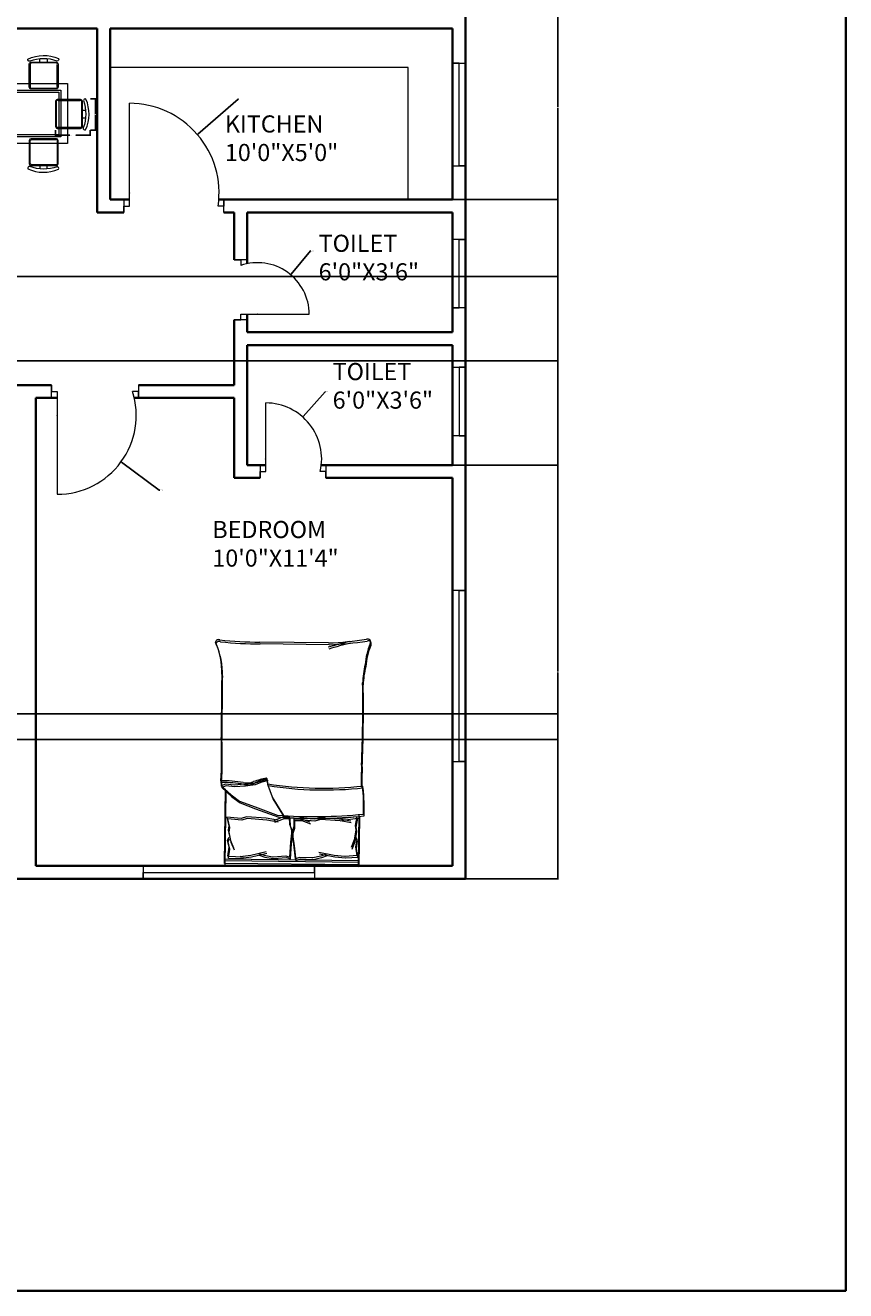
# Model space of a CAD drawing. Units: inches. Extents: x 1721 to 2510, y 1544 to 2360.
# Tile 5 of 10: x 2222 to 2510, y 1544 to 1988. Entities that reach past the tile are written whole.
import ezdxf

# ---------------------------------------------------------------- set-up
doc = ezdxf.new("R2010")
doc.units = ezdxf.units.IN
for name, color, linetype, lineweight in [('A-ANNO-DIMS', 2, 'Continuous', 18), ('A-ANNO-TTLB', 7, 'Continuous', 35), ('A-AREA-IDEN', 7, 'Continuous', 18), ('A-DOOR', 3, 'Continuous', 18), ('A-FLOR-FIXT', 9, 'Continuous', 18), ('A-FURN', 8, 'Continuous', 13), ('A-GLAZ', 4, 'Continuous', 18), ('A-WALL', 7, 'Continuous', 35)]:
    doc.layers.add(name, color=color, linetype=linetype, lineweight=lineweight)
doc.styles.get("Standard").update_dxf_attribs({"font": 'arial.ttf'})
doc.dimstyles.get("Standard").update_dxf_attribs({"dimtxt": 0.18, "dimasz": 0.18, "dimexe": 0.18, "dimexo": 0.0625, "dimgap": 0.09, "dimtad": 0, "dimtih": 1, "dimtoh": 1, "dimdec": 4, "dimzin": 0, "dimdsep": 46, "dimtxsty": 'Standard', "dimcen": 0.09, "dimadec": 0, "dimazin": 0, "dimtfac": 1, "dimtdec": 4, "dimtofl": 0, "dimtmove": 0, "dimatfit": 3, "dimfxl": 1, "dimtolj": 1, "dimtzin": 0, "dimarcsym": 0})

# ---------------------------------------------------------------- blocks, each defined once
blk = doc.blocks.new('BED-DOUBLE')
for p, q in [((39.64, 78.43), (15.52, 78.72)), ((39.64, 78.43), (15.52, 78.72)), ((39.86, 77.8), (15.74, 78.09)), ((39.86, 77.8), (15.74, 78.09)), ((1.93, 30.11), (1.99, 28.4, 3.79)), ((1.93, 30.11), (1.99, 28.4, 3.79)), ((3.5, 28.99), (1.99, 28.4)), ((3.5, 28.99), (1.99, 28.4)), ((1.99, 28.4), (5.58, 25.17)), ((1.99, 28.4), (5.58, 25.17)), ((2.15, 29.48), (2.21, 27.77, 3.79)), ((2.15, 29.48), (2.21, 27.77, 3.79)), ((3.72, 28.36), (2.21, 27.77)), ((3.72, 28.36), (2.21, 27.77)), ((2.21, 27.77), (5.8, 24.54)), ((2.21, 27.77), (5.8, 24.54)), ((3.23, 1.19), (3.55, 27.27)), ((3.23, 1.19), (3.55, 27.27)), ((3.45, 0.56), (3.76, 26.64)), ((3.45, 0.56), (3.76, 26.64)), ((6.54, 28.65), (3.5, 28.99)), ((6.54, 28.65), (3.5, 28.99)), ((6.75, 28.02), (3.72, 28.36)), ((6.75, 28.02), (3.72, 28.36)), ((10.33, 28.91), (6.54, 28.65)), ((10.33, 28.91), (6.54, 28.65)), ((10.55, 28.28), (6.75, 28.02)), ((10.55, 28.28), (6.75, 28.02)), ((13.68, 29.32), (10.33, 28.91)), ((13.68, 29.32), (10.33, 28.91)), ((13.89, 28.69), (10.55, 28.28)), ((13.89, 28.69), (10.55, 28.28)), ((15.66, 30.21), (13.68, 29.32)), ((15.66, 30.21), (13.68, 29.32)), ((15.88, 29.58), (13.89, 28.69)), ((15.88, 29.58), (13.89, 28.69)), ((18.1, 30.79), (15.66, 30.21)), ((18.1, 30.79), (15.66, 30.21)), ((18.31, 30.16), (15.88, 29.58)), ((18.31, 30.16), (15.88, 29.58)), ((18.38, 28.81), (18.1, 30.79)), ((18.38, 28.81), (18.1, 30.79)), ((18.59, 28.18), (18.31, 30.16)), ((18.59, 28.18), (18.31, 30.16)), ((20, 24.39), (18.38, 28.81)), ((20, 24.39), (18.38, 28.81)), ((20.21, 23.76), (18.59, 28.18)), ((20.21, 23.76), (18.59, 28.18)), ((5.58, 25.17), (8.44, 23.01)), ((5.58, 25.17), (8.44, 23.01)), ((5.8, 24.54), (8.66, 22.38)), ((5.8, 24.54), (8.66, 22.38)), ((8.44, 23.01), (13.88, 20.98)), ((8.44, 23.01), (13.88, 20.98)), ((8.66, 22.38), (14.1, 20.35)), ((8.66, 22.38), (14.1, 20.35)), ((24.03, 17.98), (20, 24.39)), ((24.03, 17.98), (20, 24.39)), ((24.24, 17.35), (20.21, 23.76)), ((24.24, 17.35), (20.21, 23.76)), ((13.88, 20.98), (22.02, 18)), ((13.88, 20.98), (22.02, 18)), ((14.1, 20.35), (22.24, 17.37)), ((14.1, 20.35), (22.24, 17.37)), ((50.28, 18.38), (50.07, 0.63)), ((50.28, 18.38), (50.07, 0.63)), ((50.5, 17.75), (50.29, 0)), ((50.5, 17.75), (50.29, 0)), ((9.01, 16.97), (3.98, 17.42)), ((3.98, 17.42), (4.71, 14.34)), ((9.01, 16.97), (3.98, 17.42)), ((3.98, 17.42), (4.71, 14.34)), ((9.23, 16.34), (4.2, 16.8)), ((4.2, 16.8), (4.92, 13.71)), ((9.23, 16.34), (4.2, 16.8)), ((4.2, 16.8), (4.92, 13.71)), ((4.71, 14.34), (4.5, 12.77)), ((4.71, 14.34), (4.5, 12.77)), ((4.92, 13.71), (4.72, 12.14)), ((4.92, 13.71), (4.72, 12.14)), ((10.94, 17.49), (9.01, 16.97)), ((10.94, 17.49), (9.01, 16.97)), ((11.15, 16.86), (9.23, 16.34)), ((11.15, 16.86), (9.23, 16.34)), ((17.8, 16.99), (10.94, 17.49)), ((17.8, 16.99), (10.94, 17.49)), ((18.02, 16.36), (11.15, 16.86)), ((18.02, 16.36), (11.15, 16.86)), ((21.75, 16.29), (17.8, 16.99)), ((21.75, 16.29), (17.8, 16.99)), ((21.96, 15.66), (18.02, 16.36)), ((21.96, 15.66), (18.02, 16.36)), ((23.54, 17.35), (20.51, 16.13)), ((23.54, 17.35), (20.51, 16.13)), ((23.75, 16.73), (20.73, 15.5)), ((23.75, 16.73), (20.73, 15.5)), ((25.94, 17.48), (23.54, 17.35)), ((25.94, 17.48), (23.54, 17.35)), ((26.16, 16.85), (23.75, 16.73)), ((26.16, 16.85), (23.75, 16.73)), ((26.07, 14.85), (25.94, 17.48)), ((26.07, 14.85), (25.94, 17.48)), ((26.73, 13.04), (26.07, 14.85)), ((26.73, 13.04), (26.07, 14.85)), ((26.29, 14.22), (26.16, 16.85)), ((26.29, 14.22), (26.16, 16.85)), ((26.95, 12.41), (26.29, 14.22)), ((26.95, 12.41), (26.29, 14.22)), ((27.02, 12.38), (27.61, 14.21)), ((27.02, 12.38), (27.61, 14.21)), ((27.23, 11.75), (27.82, 13.58)), ((27.23, 11.75), (27.82, 13.58)), ((27.61, 14.21), (27.64, 16.84)), ((27.61, 14.21), (27.64, 16.84)), ((27.64, 16.84), (30.05, 16.81)), ((27.64, 16.84), (30.05, 16.81)), ((27.82, 13.58), (27.85, 16.21)), ((27.82, 13.58), (27.85, 16.21)), ((27.85, 16.21), (30.26, 16.18)), ((27.85, 16.21), (30.26, 16.18)), ((34.67, 16.66), (29.65, 17.12)), ((34.67, 16.66), (29.65, 17.12)), ((34.89, 16.03), (29.86, 16.49)), ((34.89, 16.03), (29.86, 16.49)), ((30.05, 16.81), (33.11, 15.7)), ((30.05, 16.81), (33.11, 15.7)), ((30.26, 16.18), (33.33, 15.07)), ((30.26, 16.18), (33.33, 15.07)), ((36.6, 17.19), (34.67, 16.66)), ((36.6, 17.19), (34.67, 16.66)), ((36.81, 16.56), (34.89, 16.03)), ((36.81, 16.56), (34.89, 16.03)), ((43.46, 16.68), (36.6, 17.19)), ((43.46, 16.68), (36.6, 17.19)), ((43.68, 16.05), (36.81, 16.56)), ((43.68, 16.05), (36.81, 16.56)), ((43.46, 16.68), (44.58, 16.98)), ((43.46, 16.68), (44.58, 16.98)), ((47.41, 15.98), (43.46, 16.68)), ((47.41, 15.98), (43.46, 16.68)), ((43.68, 16.05), (44.79, 16.35)), ((43.68, 16.05), (44.79, 16.35)), ((47.62, 15.35), (43.68, 16.05)), ((47.62, 15.35), (43.68, 16.05)), ((44.58, 16.98), (49.58, 17.63)), ((44.58, 16.98), (49.58, 17.63)), ((44.79, 16.35), (49.8, 17)), ((44.79, 16.35), (49.8, 17)), ((49.58, 17.63), (48.98, 14.52)), ((49.58, 17.63), (48.98, 14.52)), ((48.98, 14.52), (49.24, 12.96)), ((48.98, 14.52), (49.24, 12.96)), ((49.8, 17), (49.19, 13.89)), ((49.8, 17), (49.19, 13.89)), ((49.19, 13.89), (49.46, 12.33)), ((49.19, 13.89), (49.46, 12.33)), ((4.25, 9.35), (4.77, 10.37)), ((4.25, 9.35), (4.77, 10.37)), ((4.8, 6.82), (4.25, 9.35)), ((4.8, 6.82), (4.25, 9.35)), ((4.47, 8.72), (4.98, 9.74)), ((4.47, 8.72), (4.98, 9.74)), ((4.5, 12.77), (5.25, 9.26)), ((4.5, 12.77), (5.25, 9.26)), ((4.72, 12.14), (5.46, 8.63)), ((4.72, 12.14), (5.46, 8.63)), ((5.25, 9.26), (6.37, 6.62)), ((5.25, 9.26), (6.37, 6.62)), ((26.39, 8.62), (26.8, 11.77)), ((26.39, 8.62), (26.8, 11.77)), ((26.61, 7.99), (27.01, 11.14)), ((26.61, 7.99), (27.01, 11.14)), ((26.8, 11.77), (26.73, 13.04)), ((26.8, 11.77), (26.73, 13.04)), ((27.01, 11.14), (26.95, 12.41)), ((27.01, 11.14), (26.95, 12.41)), ((27, 11.1), (27.02, 12.38)), ((27, 11.1), (27.02, 12.38)), ((27.53, 7.98), (27, 11.1)), ((27.53, 7.98), (27, 11.1)), ((27.22, 10.47), (27.23, 11.75)), ((27.22, 10.47), (27.23, 11.75)), ((27.75, 7.35), (27.22, 10.47)), ((27.75, 7.35), (27.22, 10.47)), ((48.63, 9.42), (47.61, 6.74)), ((48.63, 9.42), (47.61, 6.74)), ((49.24, 12.96), (48.63, 9.42)), ((49.24, 12.96), (48.63, 9.42)), ((49.46, 12.33), (48.85, 8.79)), ((49.46, 12.33), (48.85, 8.79)), ((49.63, 9.55), (49.07, 10.55)), ((49.63, 9.55), (49.07, 10.55)), ((49.17, 7.01), (49.63, 9.55)), ((49.17, 7.01), (49.63, 9.55)), ((49.84, 8.92), (49.29, 9.92)), ((49.84, 8.92), (49.29, 9.92)), ((49.39, 6.38), (49.84, 8.92)), ((49.39, 6.38), (49.84, 8.92)), ((4.39, 3.68), (4.8, 6.82)), ((4.39, 3.68), (4.8, 6.82)), ((5.02, 6.19), (4.47, 8.72)), ((5.02, 6.19), (4.47, 8.72)), ((4.61, 3.05), (5.02, 6.19)), ((4.61, 3.05), (5.02, 6.19)), ((5.46, 8.63), (6.59, 5.99)), ((5.46, 8.63), (6.59, 5.99)), ((12.44, 4.09), (17.76, 5.35)), ((12.44, 4.09), (17.76, 5.35)), ((12.65, 3.46), (17.98, 4.72)), ((12.65, 3.46), (17.98, 4.72)), ((15.1, 4.65), (17.12, 4.04)), ((15.1, 4.65), (17.12, 4.04)), ((26.09, 3.36), (26.39, 8.62)), ((26.09, 3.36), (26.39, 8.62)), ((26.3, 2.73), (26.61, 7.99)), ((26.3, 2.73), (26.61, 7.99)), ((28.04, 2.73), (27.53, 7.98)), ((28.04, 2.73), (27.53, 7.98)), ((28.25, 2.1), (27.75, 7.35)), ((28.25, 2.1), (27.75, 7.35)), ((41.65, 3.98), (36.28, 5.04)), ((41.65, 3.98), (36.28, 5.04)), ((38.96, 4.44), (36.97, 3.75)), ((38.96, 4.44), (36.97, 3.75)), ((48.85, 8.79), (47.82, 6.11)), ((48.85, 8.79), (47.82, 6.11)), ((49.7, 3.88), (49.17, 7.01)), ((49.7, 3.88), (49.17, 7.01)), ((49.92, 3.25), (49.39, 6.38)), ((49.92, 3.25), (49.39, 6.38)), ((50.07, 0.63), (3.23, 1.19)), ((50.07, 0.63), (3.23, 1.19)), ((50.09, 2.13), (3.25, 2.69)), ((50.09, 2.13), (3.25, 2.69)), ((50.29, 0), (3.45, 0.56)), ((50.29, 0), (3.45, 0.56)), ((50.31, 1.5), (3.47, 2.06)), ((50.31, 1.5), (3.47, 2.06)), ((4.39, 3.68), (9.69, 3.52)), ((4.39, 3.68), (9.69, 3.52)), ((4.61, 3.05), (9.9, 2.89)), ((4.61, 3.05), (9.9, 2.89)), ((8.71, 3.62), (12.44, 4.09)), ((8.71, 3.62), (12.44, 4.09)), ((9.69, 3.52), (8.71, 3.62)), ((9.69, 3.52), (8.71, 3.62)), ((8.92, 2.99), (12.65, 3.46)), ((8.92, 2.99), (12.65, 3.46)), ((9.9, 2.89), (8.92, 2.99)), ((9.9, 2.89), (8.92, 2.99)), ((15.32, 4.02), (17.34, 3.41)), ((15.32, 4.02), (17.34, 3.41)), ((17.12, 4.04), (19.98, 3.48)), ((17.12, 4.04), (19.98, 3.48)), ((17.34, 3.41), (20.2, 2.85)), ((17.34, 3.41), (20.2, 2.85)), ((19.98, 3.48), (20.3, 3.49)), ((19.98, 3.48), (20.3, 3.49)), ((20.2, 2.85), (20.52, 2.86)), ((20.2, 2.85), (20.52, 2.86)), ((20.3, 3.49), (24.64, 3.85)), ((20.3, 3.49), (24.64, 3.85)), ((20.52, 2.86), (24.86, 3.22)), ((20.52, 2.86), (24.86, 3.22)), ((24.64, 3.85), (26.09, 3.36)), ((24.64, 3.85), (26.09, 3.36)), ((24.86, 3.22), (26.3, 2.73)), ((24.86, 3.22), (26.3, 2.73)), ((29.46, 3.28), (28.04, 2.73)), ((29.46, 3.28), (28.04, 2.73)), ((29.68, 2.65), (28.25, 2.1)), ((29.68, 2.65), (28.25, 2.1)), ((33.81, 3.08), (29.46, 3.28)), ((33.81, 3.08), (29.46, 3.28)), ((34.03, 2.45), (29.68, 2.65)), ((34.03, 2.45), (29.68, 2.65)), ((34.13, 3.08), (33.81, 3.08)), ((34.13, 3.08), (33.81, 3.08)), ((34.35, 2.45), (34.03, 2.45)), ((34.35, 2.45), (34.03, 2.45)), ((36.97, 3.75), (34.13, 3.08)), ((36.97, 3.75), (34.13, 3.08)), ((37.19, 3.12), (34.35, 2.45)), ((37.19, 3.12), (34.35, 2.45)), ((41.87, 3.35), (36.49, 4.41)), ((41.87, 3.35), (36.49, 4.41)), ((39.18, 3.81), (37.19, 3.12)), ((39.18, 3.81), (37.19, 3.12)), ((45.39, 3.65), (41.65, 3.98)), ((45.39, 3.65), (41.65, 3.98)), ((45.61, 3.02), (41.87, 3.35)), ((45.61, 3.02), (41.87, 3.35)), ((45.5, 3.63), (45.39, 3.65)), ((45.5, 3.63), (45.39, 3.65)), ((49.7, 3.91), (45.5, 3.63)), ((49.7, 3.91), (45.5, 3.63)), ((45.71, 3), (45.61, 3.02)), ((45.71, 3), (45.61, 3.02)), ((49.91, 3.28), (45.71, 3)), ((49.91, 3.28), (45.71, 3))]:
    blk.add_line(p, q)
for centre, radius, start, end in [((1.08, 78.52), 1.08, 61.9736, 175.3348), ((1.08, 78.52), 1.08, 61.9736, 175.3348), ((-20.36, 68.78), 22.61, 356.7862, 25.7829), ((-20.36, 68.78), 22.61, 356.7862, 25.7829), ((1.29, 77.89), 1.08, 61.9736, 175.3348), ((1.29, 77.89), 1.08, 61.9736, 175.3348), ((-20.14, 68.15), 22.61, 356.7862, 25.7829), ((-20.14, 68.15), 22.61, 356.7862, 25.7829), ((15.63, 209.12), 130.4, 263.8146, 269.9499), ((15.63, 209.12), 130.4, 263.8146, 269.9499), ((15.85, 208.49), 130.4, 263.8146, 269.9499), ((15.85, 208.49), 130.4, 263.8146, 269.9499), ((70.08, -22.85), 104.34, 102.698, 107.0202), ((70.08, -22.85), 104.34, 102.698, 107.0202), ((34.83, 197.67), 119.34, 272.3106, 278.7239), ((34.83, 197.67), 119.34, 272.3106, 278.7239), ((70.29, -23.48), 104.34, 102.698, 107.0202), ((70.29, -23.48), 104.34, 102.698, 107.0202), ((35.05, 197.04), 119.34, 272.3106, 278.7239), ((35.05, 197.04), 119.34, 272.3106, 278.7239), ((75.53, 69.21), 23.09, 157.2899, 175.9668), ((75.53, 69.21), 23.09, 157.2899, 175.9668), ((75.75, 68.58), 23.09, 157.2899, 175.9668), ((75.75, 68.58), 23.09, 157.2899, 175.9668), ((53.35, 78.73), 1.07, 325.4884, 112.793), ((53.35, 78.73), 1.07, 325.4884, 112.793), ((53.56, 78.1), 1.07, 325.4884, 112.793), ((53.56, 78.1), 1.07, 325.4884, 112.793), ((4473.12, 14.21), 4471.22, 179.317, 179.60172), ((4473.12, 14.21), 4471.22, 179.317, 179.60172), ((4473.34, 13.58), 4471.22, 179.317, 179.60172), ((4473.34, 13.58), 4471.22, 179.317, 179.60172), ((80.6, 63.5), 29.05, 165.3797, 178.2261), ((80.6, 63.5), 29.05, 165.3797, 178.2261), ((80.81, 62.87), 29.05, 165.3797, 178.2261), ((80.81, 62.87), 29.05, 165.3797, 178.2261), ((-421.08, 55.88), 472.73, 357.5425, 1.0334), ((-421.08, 55.88), 472.73, 357.5425, 1.0334), ((-420.87, 55.25), 472.73, 357.5425, 1.0334), ((-420.87, 55.25), 472.73, 357.5425, 1.0334), ((-124.73, 38.32), 126.93, 356.294, 3.1513), ((-124.73, 38.32), 126.93, 356.294, 3.1513), ((-124.51, 37.69), 126.93, 356.294, 3.1513), ((-124.51, 37.69), 126.93, 356.294, 3.1513), ((217.81, 29.18), 166.73, 177.791, 180.323), ((217.81, 29.18), 166.73, 177.791, 180.323), ((218.03, 28.55), 166.73, 177.791, 180.323), ((218.03, 28.55), 166.73, 177.791, 180.323), ((3.1, -5.33), 35.46, 79.1911, 91.8805), ((3.1, -5.33), 35.46, 79.1911, 91.8805), ((3.31, -5.96), 35.46, 79.1911, 91.8805), ((3.31, -5.96), 35.46, 79.1911, 91.8805), ((11.02, 35.47), 6.1, 257.9756, 293.0532), ((11.02, 35.47), 6.1, 257.9756, 293.0532), ((11.23, 34.84), 6.1, 257.9756, 293.0532), ((11.23, 34.84), 6.1, 257.9756, 293.0532), ((22.96, 2.41), 29.06, 99.9765, 109.1954), ((22.96, 2.41), 29.06, 99.9765, 109.1954), ((23.18, 1.78), 29.06, 99.9765, 109.1954), ((23.18, 1.78), 29.06, 99.9765, 109.1954), ((17.93, 30.85), 0.181, 339.5612, 90.4525), ((17.93, 30.85), 0.181, 339.5612, 90.4525), ((18.15, 30.22), 0.181, 339.5612, 90.4525), ((18.15, 30.22), 0.181, 339.5612, 90.4525), ((37.91, 154), 126.46, 261.0993, 276.2154), ((37.91, 154), 126.46, 261.0993, 276.2154), ((38.12, 153.37), 126.46, 261.0993, 276.2154), ((38.12, 153.37), 126.46, 261.0993, 276.2154), ((-29.75, 21.28), 81.65, 358.0366, 4.9188), ((-29.75, 21.28), 81.65, 358.0366, 4.9188), ((-29.53, 20.65), 81.65, 358.0366, 4.9188), ((-29.53, 20.65), 81.65, 358.0366, 4.9188), ((34.68, 179.26), 161.69, 265.4014, 276.097), ((34.68, 179.26), 161.69, 265.4014, 276.097), ((34.89, 178.63), 161.69, 265.4014, 276.097), ((34.89, 178.63), 161.69, 265.4014, 276.097)]:
    blk.add_arc(centre, radius, start, end)
blk = doc.blocks.new('WIN-60IN-A')
for p, q in [((4.5, 60), (0, 60)), ((2.25, 0), (2.25, 60)), ((2.25, 60), (4.5, 60)), ((4.5, 0), (0, 0)), ((0, 0), (2.25, 0))]:
    blk.add_line(p, q)
blk = doc.blocks.new('WIN-24IN-A')
for p, q in [((4.5, 24), (0, 24)), ((0, 24), (2.25, 24)), ((2.25, 24), (2.25, 0)), ((4.5, 0), (0, 0)), ((2.25, 0), (4.5, 0))]:
    blk.add_line(p, q)
blk = doc.blocks.new('WIN-24IN-B')
for p, q in [((0, 24), (4.5, 24)), ((4.5, 24), (2.25, 24)), ((2.25, 24), (2.25, 0)), ((4.5, 0), (0, 0)), ((2.25, 0), (4.5, 0))]:
    blk.add_line(p, q)
blk = doc.blocks.new('WIN-60IN-B')
for p, q in [((2.25, 60), (0, 60)), ((0, 60), (4.5, 60)), ((2.25, 0), (2.25, 60)), ((4.5, 0), (0, 0)), ((0, 0), (2.25, 0))]:
    blk.add_line(p, q)
blk = doc.blocks.new('WIN-36IN-A')
for p, q in [((2.25, 36), (0, 36)), ((0, 36), (4.5, 36)), ((2.25, 0), (2.25, 36)), ((0, 0), (4.5, 0)), ((4.5, 0), (2.25, 0))]:
    blk.add_line(p, q)
blk = doc.blocks.new('TABLE-DINING-RECT')
for points in [[(0, 21.04), (35.07, 21.04), (35.07, 0), (0, 0)], [(2.34, 18.71), (32.73, 18.71), (32.73, 2.34), (2.34, 2.34)], [(3.04, 18), (32.03, 18), (32.03, 3.04), (3.04, 3.04)]]:
    blk.add_lwpolyline(points, close=True)
blk = doc.blocks.new('CHAIR-DINING-D')
for points in [[(0.75, 9.71, -0.578392), (0.03, 10.5, -0.214524), (10.81, 10.65, -0.552014), (10.31, 9.78, 0.175809), (0.75, 9.71)], [(10.03, 9.4, -0.414214), (10.65, 8.78), (10.65, 0.62, -0.414214), (10.03, 0), (1.16, 0, -0.414214), (0.54, 0.62), (0.54, 8.78, -0.414214), (1.16, 9.4), (10.03, 9.4)], [(4.27, 9.4), (4.27, 10.52, 0.064759)]]:
    blk.add_lwpolyline(points, format="xyb")
blk.add_lwpolyline([(10.02, 9.12), (1.44, 9.12, 0.414214), (0.82, 8.5), (0.82, 0.9, 0.414214), (1.44, 0.28), (10.02, 0.28, 0.512069), (10.37, 0.9), (10.37, 8.5, 0.512069)], format="xyb", close=True)
blk.add_lwpolyline([(6.76, 10.54), (6.76, 9.4)])
blk = doc.blocks.new('CHAIR-DINING-E')
for points in [[(9.4, 10.03, 0.414214), (8.77, 10.65), (0.62, 10.65, 0.414214), (0, 10.03), (0, 1.16, 0.414214), (0.62, 0.54), (8.77, 0.54, 0.414214), (9.4, 1.16), (9.4, 10.03)], [(9.78, 10.31, -0.175809), (9.71, 0.75, 0.578392), (10.5, 0.03, 0.214524), (10.65, 10.81, 0.552014), (9.78, 10.31, -0.065079)], [(9.4, 4.27), (10.52, 4.27, -0.064759)]]:
    blk.add_lwpolyline(points, format="xyb")
blk.add_lwpolyline([(9.12, 10.02), (9.12, 1.44, -0.414214), (8.5, 0.82), (0.9, 0.82, -0.414214), (0.28, 1.44), (0.28, 10.02, -0.512069), (0.9, 10.37), (8.5, 10.37, -0.512069)], format="xyb", close=True)
blk.add_lwpolyline([(10.54, 6.76), (9.4, 6.76)])
blk = doc.blocks.new('*D38')
at = {"layer": 'A-ANNO-DIMS', "color": 0, "lineweight": -2, "transparency": 16777216}
for p, q in [((2232.9, 1950.95), (2232.9, 1949.01)), ((2233.08, 1949.19), (2237.9, 1949.19)), ((2244.86, 1949.19), (2240.04, 1949.19)), ((2245.04, 1950.95), (2245.04, 1949.01))]:
    blk.add_line(p, q, dxfattribs=at)
at = {"layer": 'A-ANNO-DIMS', "color": 0, "transparency": 16777216}
for points in [[(2233.08, 1949.22), (2233.08, 1949.16), (2232.9, 1949.19)], [(2244.86, 1949.22), (2244.86, 1949.16), (2245.04, 1949.19)]]:
    blk.add_solid(points, dxfattribs=at)
at = {"layer": 'Defpoints', "color": 0, "transparency": 16777216}
for p in [(2232.9, 1951.01), (2245.04, 1951.01), (2245.04, 1949.19)]:
    blk.add_point(p, dxfattribs=at)
at = {"layer": 'A-ANNO-DIMS', "color": 0, "transparency": 16777216, "insert": (2238.97, 1949.19), "char_height": 0.18, "attachment_point": 5}
blk.add_mtext('\\A1;CHAIR E 12 TYP.', dxfattribs=at)
blk = doc.blocks.new('*D39')
at = {"layer": 'A-ANNO-DIMS', "color": 0, "lineweight": -2, "transparency": 16777216}
for p, q in [((2245.11, 1961.95), (2247.05, 1961.95)), ((2246.87, 1961.77), (2246.87, 1956.66)), ((2246.87, 1951.19), (2246.87, 1956.3)), ((2245.11, 1951.01), (2247.05, 1951.01))]:
    blk.add_line(p, q, dxfattribs=at)
at = {"layer": 'A-ANNO-DIMS', "color": 0, "transparency": 16777216}
for points in [[(2246.84, 1961.77), (2246.9, 1961.77), (2246.87, 1961.95)], [(2246.84, 1951.19), (2246.9, 1951.19), (2246.87, 1951.01)]]:
    blk.add_solid(points, dxfattribs=at)
at = {"layer": 'Defpoints', "color": 0, "transparency": 16777216}
for p in [(2245.04, 1961.95), (2246.87, 1961.95), (2245.04, 1951.01)]:
    blk.add_point(p, dxfattribs=at)
at = {"layer": 'A-ANNO-DIMS', "color": 0, "transparency": 16777216, "insert": (2246.87, 1956.48), "char_height": 0.18, "attachment_point": 5}
blk.add_mtext('\\A1;11 TYP.', dxfattribs=at)
blk = doc.blocks.new('*D50')
at = {"layer": 'A-ANNO-DIMS', "color": 0, "lineweight": -2, "transparency": 16777216}
for p, q in [((2372.06, 1991.13), (2409.08, 1991.13)), ((2408.9, 1990.95), (2408.9, 1959.06)), ((2408.9, 1926.81), (2408.9, 1958.7)), ((2372.06, 1926.63), (2409.08, 1926.63))]:
    blk.add_line(p, q, dxfattribs=at)
at = {"layer": 'A-ANNO-DIMS', "color": 0, "transparency": 16777216}
for points in [[(2408.87, 1990.95), (2408.93, 1990.95), (2408.9, 1991.13)], [(2408.87, 1926.81), (2408.93, 1926.81), (2408.9, 1926.63)]]:
    blk.add_solid(points, dxfattribs=at)
at = {"layer": 'Defpoints', "color": 0, "transparency": 16777216}
for p in [(2372, 1991.13), (2408.9, 1991.13), (2372, 1926.63)]:
    blk.add_point(p, dxfattribs=at)
at = {"layer": 'A-ANNO-DIMS', "color": 0, "transparency": 16777216, "insert": (2408.9, 1958.88), "char_height": 0.18, "attachment_point": 5}
blk.add_mtext('\\A1;64.5', dxfattribs=at)
blk = doc.blocks.new('*D51')
at = {"layer": 'A-ANNO-DIMS', "color": 0, "lineweight": -2, "transparency": 16777216}
for p, q in [((2372.06, 1926.63), (2409.08, 1926.63)), ((2408.9, 1926.45), (2408.9, 1880.31)), ((2408.9, 1833.81), (2408.9, 1879.95)), ((2372.06, 1833.63), (2409.08, 1833.63))]:
    blk.add_line(p, q, dxfattribs=at)
at = {"layer": 'A-ANNO-DIMS', "color": 0, "transparency": 16777216}
for points in [[(2408.87, 1926.45), (2408.93, 1926.45), (2408.9, 1926.63)], [(2408.87, 1833.81), (2408.93, 1833.81), (2408.9, 1833.63)]]:
    blk.add_solid(points, dxfattribs=at)
at = {"layer": 'Defpoints', "color": 0, "transparency": 16777216}
for p in [(2372, 1926.63), (2408.9, 1926.63), (2372, 1833.63)]:
    blk.add_point(p, dxfattribs=at)
at = {"layer": 'A-ANNO-DIMS', "color": 0, "transparency": 16777216, "insert": (2408.9, 1880.13), "char_height": 0.18, "attachment_point": 5}
blk.add_mtext('\\A1;93', dxfattribs=at)
blk = doc.blocks.new('*D52')
at = {"layer": 'A-ANNO-DIMS', "color": 0, "lineweight": -2, "transparency": 16777216}
for p, q in [((2372.06, 1833.63), (2409.08, 1833.63)), ((2408.9, 1833.45), (2408.9, 1761.31)), ((2408.9, 1688.81), (2408.9, 1760.95)), ((2376.56, 1688.63), (2409.08, 1688.63))]:
    blk.add_line(p, q, dxfattribs=at)
at = {"layer": 'A-ANNO-DIMS', "color": 0, "transparency": 16777216}
for points in [[(2408.87, 1833.45), (2408.93, 1833.45), (2408.9, 1833.63)], [(2408.87, 1688.81), (2408.93, 1688.81), (2408.9, 1688.63)]]:
    blk.add_solid(points, dxfattribs=at)
at = {"layer": 'Defpoints', "color": 0, "transparency": 16777216}
for p in [(2372, 1833.63), (2408.9, 1833.63), (2376.5, 1688.63)]:
    blk.add_point(p, dxfattribs=at)
at = {"layer": 'A-ANNO-DIMS', "color": 0, "transparency": 16777216, "insert": (2408.9, 1761.13), "char_height": 0.18, "attachment_point": 5}
blk.add_mtext('\\A1;145', dxfattribs=at)
blk = doc.blocks.new('*D54')
at = {"layer": 'A-ANNO-DIMS', "color": 0, "lineweight": -2, "transparency": 16777216}
for p, q in [((2047.06, 1746.49), (2409.08, 1746.49)), ((2408.9, 1746.31), (2408.9, 1742.17)), ((2408.9, 1737.67), (2408.9, 1741.81)), ((2047.06, 1737.49), (2409.08, 1737.49))]:
    blk.add_line(p, q, dxfattribs=at)
at = {"layer": 'A-ANNO-DIMS', "color": 0, "transparency": 16777216}
for points in [[(2408.87, 1746.31), (2408.93, 1746.31), (2408.9, 1746.49)], [(2408.87, 1737.67), (2408.93, 1737.67), (2408.9, 1737.49)]]:
    blk.add_solid(points, dxfattribs=at)
at = {"layer": 'Defpoints', "color": 0, "transparency": 16777216}
for p in [(2047, 1746.49), (2408.9, 1746.49), (2047, 1737.49)]:
    blk.add_point(p, dxfattribs=at)
at = {"layer": 'A-ANNO-DIMS', "color": 0, "transparency": 16777216, "insert": (2408.9, 1741.99), "char_height": 0.18, "attachment_point": 5}
blk.add_mtext('\\A1;9', dxfattribs=at)
blk = doc.blocks.new('*D58')
at = {"layer": 'A-ANNO-DIMS', "color": 0, "lineweight": -2, "transparency": 16777216}
for p, q in [((2042.56, 1899.66), (2409.08, 1899.66)), ((2408.9, 1899.48), (2408.9, 1885.09)), ((2408.9, 1870.34), (2408.9, 1884.73)), ((2042.56, 1870.16), (2409.08, 1870.16))]:
    blk.add_line(p, q, dxfattribs=at)
at = {"layer": 'A-ANNO-DIMS', "color": 0, "transparency": 16777216}
for points in [[(2408.87, 1899.48), (2408.93, 1899.48), (2408.9, 1899.66)], [(2408.87, 1870.34), (2408.93, 1870.34), (2408.9, 1870.16)]]:
    blk.add_solid(points, dxfattribs=at)
at = {"layer": 'Defpoints', "color": 0, "transparency": 16777216}
for p in [(2042.5, 1899.66), (2408.9, 1899.66), (2042.5, 1870.16)]:
    blk.add_point(p, dxfattribs=at)
at = {"layer": 'A-ANNO-DIMS', "color": 0, "transparency": 16777216, "insert": (2408.9, 1884.91), "char_height": 0.18, "attachment_point": 5}
blk.add_mtext('\\A1;29.505', dxfattribs=at)
blk = doc.blocks.new('*D77')
at = {"layer": 'A-ANNO-DIMS', "color": 0, "lineweight": -2, "transparency": 16777216}
for p, q in [((2296.82, 1961.81), (2282.69, 1949.61)), ((2297, 1961.81), (2296.82, 1961.81)), ((2258.68, 1928.97), (2258.86, 1928.97)), ((2258.77, 1928.88), (2258.77, 1929.06))]:
    blk.add_line(p, q, dxfattribs=at)
at = {"layer": 'A-ANNO-DIMS', "color": 0, "transparency": 16777216}
blk.add_solid([(2282.67, 1949.63), (2282.71, 1949.59), (2282.55, 1949.49)], dxfattribs=at)
at = {"layer": 'Defpoints', "color": 0, "transparency": 16777216}
for p in [(2282.55, 1949.49), (2258.77, 1928.97)]:
    blk.add_point(p, dxfattribs=at)
at = {"layer": 'A-ANNO-DIMS', "color": 0, "transparency": 16777216, "insert": (2297.46, 1961.81), "char_height": 0.18, "attachment_point": 5}
blk.add_mtext('\\A1;R31.41', dxfattribs=at)
blk = doc.blocks.new('*D81')
at = {"layer": 'A-ANNO-DIMS', "color": 0, "lineweight": -2, "transparency": 16777216}
for p, q in [((2233.41, 1851.06), (2233.59, 1851.06)), ((2233.5, 1850.97), (2233.5, 1851.15)), ((2269.22, 1824.87), (2255.97, 1834.58)), ((2269.4, 1824.87), (2269.22, 1824.87))]:
    blk.add_line(p, q, dxfattribs=at)
at = {"layer": 'A-ANNO-DIMS', "color": 0, "transparency": 16777216}
blk.add_solid([(2255.99, 1834.61), (2255.95, 1834.56), (2255.83, 1834.69)], dxfattribs=at)
at = {"layer": 'Defpoints', "color": 0, "transparency": 16777216}
for p in [(2233.5, 1851.06), (2255.83, 1834.69)]:
    blk.add_point(p, dxfattribs=at)
at = {"layer": 'A-ANNO-DIMS', "color": 0, "transparency": 16777216, "insert": (2269.95, 1824.87), "char_height": 0.18, "attachment_point": 5}
blk.add_mtext('\\A1;R27.684', dxfattribs=at)
blk = doc.blocks.new('*D92')
at = {"layer": 'A-ANNO-DIMS', "color": 0, "lineweight": -2, "transparency": 16777216}
for p, q in [((2322.21, 1908.64), (2315.39, 1900.46)), ((2322.39, 1908.64), (2322.21, 1908.64)), ((2303.61, 1886.47), (2303.79, 1886.47)), ((2303.7, 1886.38), (2303.7, 1886.56))]:
    blk.add_line(p, q, dxfattribs=at)
at = {"layer": 'A-ANNO-DIMS', "color": 0, "transparency": 16777216}
blk.add_solid([(2315.36, 1900.48), (2315.41, 1900.45), (2315.27, 1900.33)], dxfattribs=at)
at = {"layer": 'Defpoints', "color": 0, "transparency": 16777216}
for p in [(2315.27, 1900.33), (2303.7, 1886.47)]:
    blk.add_point(p, dxfattribs=at)
at = {"layer": 'A-ANNO-DIMS', "color": 0, "transparency": 16777216, "insert": (2322.87, 1908.64), "char_height": 0.18, "attachment_point": 5}
blk.add_mtext('\\A1;R18.05', dxfattribs=at)
blk = doc.blocks.new('*D93')
at = {"layer": 'A-ANNO-DIMS', "color": 0, "lineweight": -2, "transparency": 16777216}
for p, q in [((2327.32, 1859.27), (2319.63, 1850.58)), ((2327.5, 1859.27), (2327.32, 1859.27)), ((2306.41, 1835.75), (2306.59, 1835.75)), ((2306.5, 1835.66), (2306.5, 1835.84))]:
    blk.add_line(p, q, dxfattribs=at)
at = {"layer": 'A-ANNO-DIMS', "color": 0, "transparency": 16777216}
blk.add_solid([(2319.61, 1850.6), (2319.65, 1850.56), (2319.51, 1850.45)], dxfattribs=at)
at = {"layer": 'Defpoints', "color": 0, "transparency": 16777216}
for p in [(2319.51, 1850.45), (2306.5, 1835.75)]:
    blk.add_point(p, dxfattribs=at)
at = {"layer": 'A-ANNO-DIMS', "color": 0, "transparency": 16777216, "insert": (2327.98, 1859.27), "char_height": 0.18, "attachment_point": 5}
blk.add_mtext('\\A1;R19.63', dxfattribs=at)

msp = doc.modelspace()

# ---------------------------------------------------------------- linework, layer by layer
at = {"layer": 'A-ANNO-TTLB'}
msp.add_lwpolyline([(1721.1268, 2360.2177), (2509.707, 2360.2177), (2509.707, 1544.3037), (1721.1268, 1544.3037)], close=True, dxfattribs=at)
at = {"layer": 'A-DOOR'}
for p, q in [((2258.7732, 1924.3798), (2258.7732, 1960.3798)), ((2256.7732, 1926.6298), (2256.7732, 1922.1298)), ((2291.8439, 1922.1298), (2291.8439, 1926.6298)), ((2291.8439, 1926.6298), (2291.8439, 1924.3798)), ((2256.7732, 1922.1298), (2256.7732, 1924.3798)), ((2256.7732, 1924.3798), (2258.7732, 1924.3798)), ((2291.8439, 1924.3798), (2289.8439, 1924.3798)), ((2300.0024, 1905.5119), (2295.5024, 1905.5119)), ((2295.5024, 1905.5119), (2297.7524, 1905.5119)), ((2297.7524, 1905.5119), (2297.7524, 1903.5119)), ((2297.7524, 1884.4729), (2297.7524, 1886.4729)), ((2297.7524, 1886.4729), (2321.7524, 1886.4729)), ((2300.0024, 1884.4729), (2295.5024, 1884.4729)), ((2295.5024, 1884.4729), (2297.7524, 1884.4729)), ((2231.5043, 1857.1298), (2231.5043, 1861.6298)), ((2231.5043, 1861.6298), (2231.5043, 1859.3798)), ((2231.5043, 1859.3798), (2233.5043, 1859.3798)), ((2233.5043, 1859.3798), (2233.5043, 1823.3798)), ((2261.9091, 1859.3798), (2259.9091, 1859.3798)), ((2261.9091, 1861.6298), (2261.9091, 1857.1298)), ((2261.9091, 1857.1298), (2261.9091, 1859.3798)), ((2261.9091, 1857.1298), (2261.9091, 1857.1298)), ((2306.5787, 1831.3798), (2306.5787, 1855.3798)), ((2304.5787, 1833.6298), (2304.5787, 1829.1298)), ((2304.5787, 1829.1298), (2304.5787, 1831.3798)), ((2304.5787, 1831.3798), (2306.5787, 1831.3798)), ((2327.6364, 1831.3798), (2325.6364, 1831.3798)), ((2327.6364, 1833.6298), (2327.6364, 1829.1298)), ((2327.6364, 1829.1298), (2327.6364, 1831.3798))]:
    msp.add_line(p, q, dxfattribs=at)
for centre, radius, start, end in [((2258.7732, 1928.9716), 31.4082, 351.593363, 90), ((2303.7039, 1886.4729), 18.0485, 0, 109.253461), ((2233.5043, 1851.0633), 27.6835, 270, 17.482379), ((2306.4972, 1835.7485), 19.6314, 347.141912, 89.762205)]:
    msp.add_arc(centre, radius, start, end, dxfattribs=at)
at = {"layer": 'A-FLOR-FIXT'}
for p, q in [((2356.3864, 1972.8786), (2252.0024, 1972.8786)), ((2356.3864, 1926.6298), (2356.3864, 1972.8786))]:
    msp.add_line(p, q, dxfattribs=at)
at = {"layer": 'A-FURN'}
for points in [[(2233.1795, 1938.5415, 0.41421356), (2233.7999, 1939.1619), (2233.7999, 1947.3164, 0.41421356), (2233.1795, 1947.9368), (2224.3109, 1947.9368, 0.41421356), (2223.6905, 1947.3164), (2223.6905, 1939.1619, 0.41421356), (2224.3109, 1938.5415), (2233.1795, 1938.5415)], [(2233.4585, 1938.1581, -0.17580928), (2223.9057, 1938.2304, 0.57839206), (2223.1819, 1937.4346, 0.21452438), (2233.9651, 1937.29, 0.55201397), (2233.4585, 1938.1581, -0.06507904)], [(2227.426, 1938.5415), (2227.426, 1937.4199, -0.06475861)]]:
    msp.add_lwpolyline(points, format="xyb", dxfattribs=at)
msp.add_lwpolyline([(2233.1757, 1938.821), (2224.5905, 1938.821, -0.41421356), (2223.97, 1939.4414), (2223.97, 1947.0369, -0.41421356), (2224.5905, 1947.6573), (2233.1757, 1947.6573, -0.51206948), (2233.5204, 1947.0369), (2233.5204, 1939.4414, -0.51206948)], format="xyb", close=True, dxfattribs=at)
msp.add_lwpolyline([(2229.9084, 1937.3995), (2229.9084, 1938.5415)], dxfattribs=at)
at = {"layer": 'A-WALL'}
for p, q in [((2376.5024, 2285.1298), (2376.5024, 1688.6298)), ((2247.5024, 1986.6298), (2132.0024, 1986.6298)), ((2132.0024, 1986.6298), (2247.5024, 1986.6298)), ((2247.5024, 1922.1298), (2247.5024, 1986.6298)), ((2252.0024, 1986.6298), (2372.0024, 1986.6298)), ((2252.0024, 1986.6298), (2252.0024, 1926.6298)), ((2372.0024, 1986.6298), (2372.0024, 1926.6298)), ((2252.0024, 1926.6298), (2258.7732, 1926.6298)), ((2290.094, 1926.6298), (2372.0024, 1926.6298)), ((2372.0024, 1926.6298), (2300.0024, 1926.6298)), ((2252.0024, 1922.1298), (2247.5024, 1922.1298)), ((2247.5024, 1922.1298), (2256.7732, 1922.1298)), ((2291.8439, 1922.1298), (2295.5024, 1922.1298)), ((2295.5024, 1905.5119), (2295.5024, 1922.1298)), ((2300.0024, 1922.1298), (2300.0024, 1904.1378)), ((2300.0024, 1922.1298), (2372.0024, 1922.1298)), ((2372.0024, 1922.1298), (2372.0024, 1880.1298)), ((2300.0024, 1886.4729), (2300.0024, 1880.1298)), ((2295.5024, 1861.6298), (2295.5024, 1884.4729)), ((2300.0024, 1880.1298), (2372.0024, 1880.1298)), ((2300.0024, 1875.6298), (2372.0024, 1875.6298)), ((2300.0024, 1875.6298), (2300.0024, 1833.6298)), ((2372.0024, 1875.6298), (2372.0024, 1833.6298)), ((2231.5043, 1861.6298), (2216.0057, 1861.6298)), ((2295.5024, 1861.6298), (2261.9091, 1861.6298)), ((2226.0024, 1857.1298), (2226.0024, 1693.1298)), ((2226.0024, 1857.1298), (2233.5043, 1857.1298)), ((2260.5149, 1857.1298), (2295.5024, 1857.1298)), ((2295.5024, 1829.1298), (2295.5024, 1857.1298)), ((2300.0024, 1833.6298), (2306.5787, 1833.6298)), ((2326.014, 1833.6298), (2372.0024, 1833.6298)), ((2300.0024, 1829.1298), (2295.5024, 1829.1298)), ((2295.5024, 1829.1298), (2304.5787, 1829.1298)), ((2327.6364, 1829.1298), (2372.0024, 1829.1298)), ((2372.0024, 1829.1298), (2372.0024, 1693.1298)), ((2226.0024, 1693.1298), (2372.0024, 1693.1298)), ((1798.0024, 1688.6298), (2376.5024, 1688.6298))]:
    msp.add_line(p, q, dxfattribs=at)

# ---------------------------------------------------------------- block references
at = {"layer": 'A-FURN'}
for name, p in [('CHAIR-DINING-D', (2223.1531, 1965.3944)), ('TABLE-DINING-RECT', (2201.9727, 1946.2562)), ('CHAIR-DINING-E', (2232.9011, 1951.0484)), ('BED-DOUBLE', (2288.8961, 1692.8498))]:
    msp.add_blockref(name, p, dxfattribs=at)
at = {"layer": 'A-GLAZ'}
for name, p in [('WIN-36IN-A', (2372.002, 1938.488)), ('WIN-24IN-B', (2372.002, 1843.8704))]:
    msp.add_blockref(name, p, dxfattribs=at)
at = {"layer": 'A-GLAZ', "extrusion": (0, 0, -1), "zscale": -1}
for name, p, rotation in [('WIN-24IN-A', (-2372.002, 1912.7125), 180), ('WIN-60IN-A', (-2263.5643, 1688.6294), 90)]:
    msp.add_blockref(name, p, dxfattribs=dict(at, rotation=rotation))
msp.add_blockref('WIN-60IN-B', (-2376.5028, 1729.6983), dxfattribs=at)

# ---------------------------------------------------------------- texts
at = {"layer": 'A-AREA-IDEN', "char_height": 6, "attachment_point": 1}
for s, width, insert in [('KITCHEN\\P10\'0"X5\'0"', 134.37007, (2292.2133, 1956.1439)), ('TOILET\\P6\'0"X3\'6"', 38.352957, (2325.0687, 1914.3275)), ('TOILET\\P6\'0"X3\'6"', 72.302642, (2329.9749, 1869.3776)), ('BEDROOM\\P10\'0"X11\'4"', 132.065132, (2287.822, 1814.0215))]:
    msp.add_mtext_dynamic_manual_height_columns(s, width=width, gutter_width=12.5, heights=[0], dxfattribs=dict(at, insert=insert))

# ---------------------------------------------------------------- dimensions: what is measured, and where the dimension line sits
at = {"layer": 'A-ANNO-DIMS'}
for base, p1, p2, override, picture, middle in [((2408.9024, 1991.1298), (2372.0024, 1926.6298), (2372.0024, 1991.1298), {"dimdec": 1, "dimlfac": 1, "dimrnd": 0, "dimzin": 0, "dimdsep": 46, "dimlunit": 2}, '*D50', (2408.9024, 1958.8798)), ((2408.9024, 1926.6298), (2372.0024, 1833.6298), (2372.0024, 1926.6298), {"dimdec": 0, "dimlfac": 1, "dimrnd": 0, "dimzin": 0, "dimdsep": 46, "dimlunit": 2}, '*D51', (2408.9024, 1880.1298)), ((2408.9024, 1899.6648), (2042.5024, 1870.1595), (2042.5024, 1899.6648), {"dimdec": 3, "dimlfac": 1, "dimrnd": 0, "dimzin": 0, "dimdsep": 46, "dimlunit": 2}, '*D58', (2408.9024, 1884.9121)), ((2408.9024, 1833.6298), (2376.5024, 1688.6298), (2372.0024, 1833.6298), {"dimdec": 0, "dimlfac": 1, "dimrnd": 0, "dimzin": 0, "dimdsep": 46, "dimlunit": 2}, '*D52', (2408.9024, 1761.1298)), ((2408.9024, 1746.4881), (2047.0024, 1737.4881), (2047.0024, 1746.4881), {"dimdec": 0, "dimlfac": 1, "dimrnd": 0, "dimzin": 0, "dimdsep": 46, "dimlunit": 2}, '*D54', (2408.9024, 1741.9881))]:
    dim = msp.add_linear_dim(base=base, p1=p1, p2=p2, angle=90, dimstyle='Standard', override=override, dxfattribs=at)
    dim.commit()
    dim.dimension.update_dxf_attribs({"geometry": picture, "text_midpoint": middle})
dim = msp.add_linear_dim(base=(2246.8654, 1961.9548), p1=(2245.044, 1951.0094), p2=(2245.044, 1961.9548), angle=90, text='<> TYP.', dimstyle='Standard', override={"dimdec": 0, "dimlfac": 1, "dimrnd": 0, "dimzin": 0, "dimdsep": 46, "dimlunit": 2}, dxfattribs=at)
dim.commit()
dim.dimension.update_dxf_attribs({"geometry": '*D39', "text_midpoint": (2246.8654, 1956.4821)})
for center, mpoint, override, picture, middle in [((2258.7732, 1928.9716), (2282.5501, 1949.4931), {"dimdec": 2, "dimlfac": 1, "dimrnd": 0, "dimzin": 0, "dimdsep": 46, "dimlunit": 2}, '*D77', (2297.4588, 1961.806)), ((2303.7039, 1886.4729), (2315.2725, 1900.3263), {"dimdec": 2, "dimlfac": 1, "dimrnd": 0, "dimzin": 0, "dimdsep": 46, "dimlunit": 2}, '*D92', (2322.8741, 1908.6383)), ((2306.4972, 1835.7485), (2319.5105, 1850.4471), {"dimdec": 2, "dimlfac": 1, "dimrnd": 0, "dimzin": 0, "dimdsep": 46, "dimlunit": 2}, '*D93', (2327.9783, 1859.2663)), ((2233.50426, 1851.06333), (2255.82681, 1834.69014), {"dimdec": 3, "dimlfac": 1, "dimrnd": 0, "dimzin": 0, "dimdsep": 46, "dimlunit": 2}, '*D81', (2269.94973, 1824.86623))]:
    dim = msp.add_radius_dim(center=center, mpoint=mpoint, dimstyle='Standard', override=override, dxfattribs=at)
    dim.commit()
    dim.dimension.update_dxf_attribs({"geometry": picture, "text_midpoint": middle, "dimtype": 164})
dim = msp.add_linear_dim(base=(2245.044, 1949.188), p1=(2232.901, 1951.0094), p2=(2245.044, 1951.0094), text='CHAIR E <> TYP.', dimstyle='Standard', override={"dimdec": 0, "dimlfac": 1, "dimrnd": 0, "dimzin": 0, "dimdsep": 46, "dimlunit": 2}, dxfattribs=at)
dim.commit()
dim.dimension.update_dxf_attribs({"geometry": '*D38', "text_midpoint": (2238.9725, 1949.188)})

doc.saveas('drawing.dxf')
